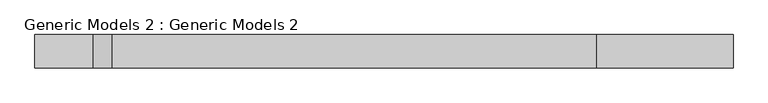
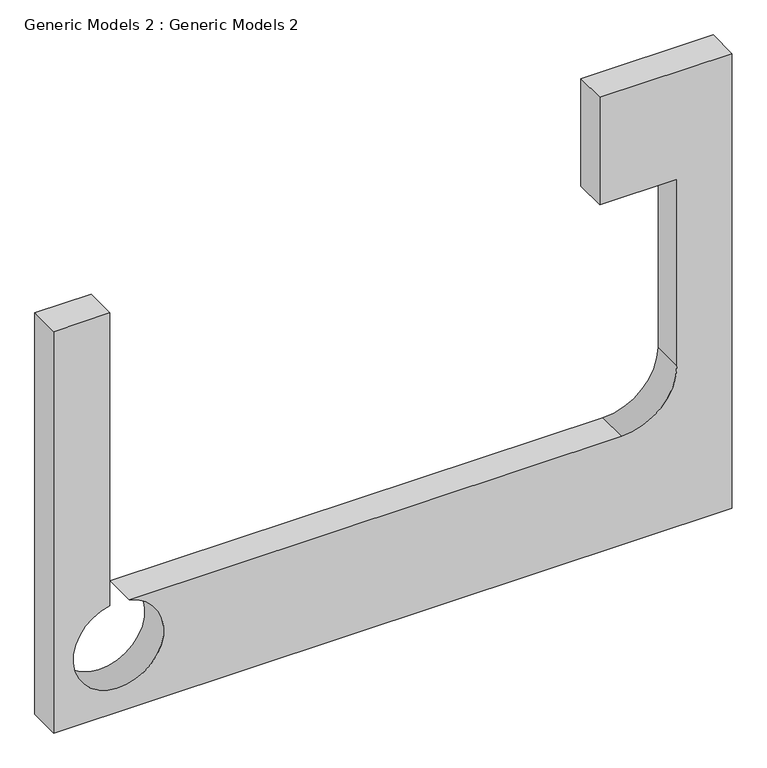
"""IFC4 building model written with IfcOpenShell, lengths in millimetres: proxy geometry, Generic Models 2 : Generic Models 2."""

from ifc_helpers import new_model, si_unit, point, frame, frame_2d, origin, place, context, project, spatial, polyline, circle_curve, trimmed, segment, composite_curve, outline, extrude, source, transform, mapped, element, save


def generic_models_2_generic_models_2_d1d1e900(model_context):
    return source(origin(), model_context, "Body", "SweptSolid", [
        extrude(outline(composite_curve([segment(polyline([(3590.0722399, -13997.6335986), (8094.058524, -13997.6335986), (8094.058524, -15237.8356484), (7030.1491239, -15237.8356484), (7030.1491239, -14513.9356484), (5181.0005, -14513.9356484)]), True, "CONTINUOUS"), segment(trimmed(circle_curve(frame_2d((5181.0005, -15030.2376981)), 516.3020498), [point((5181.0005, -14513.9356484))], [point((4664.6984502, -15030.2376981))], True, "CARTESIAN"), True, "CONTINUOUS"), segment(polyline([(4664.6984502, -15030.2376981), (4664.6984502, -19650.0519369)]), True, "CONTINUOUS"), segment(trimmed(circle_curve(frame_2d((4250.8135385, -19749.3127095)), 425.6212178), [point((4664.6984502, -19650.0519369))], [point((4668.8984575, -19829.0524212))], True, "CARTESIAN"), True, "CONTINUOUS"), segment(polyline([(4668.8984575, -19829.0524212), (7566.4335715, -19829.0524212), (7566.4335715, -20355.9358231), (3590.0722399, -20355.9358231), (3590.0722399, -13997.6335986)]), True, "CONTINUOUS")], self_intersect=False)), frame((0.0, -4597.9088252, 0.0), z_axis=(0.0, 1.0, 0.0), x_axis=(0.0, 0.0, 1.0)), (0.0, 0.0, 1.0), 304.8),
    ])


if __name__ == "__main__":
    model = new_model("IFC4")
    model_context = context("Model", 3, world=origin())
    ifc_project = project(units=[si_unit("LENGTHUNIT", "METRE", prefix="MILLI")], contexts=[model_context])
    site = spatial("IfcSite", under=ifc_project)
    building = spatial("IfcBuilding", under=site)
    placement = place(None, origin())
    generic_models_2_generic_models_2_shape = generic_models_2_generic_models_2_d1d1e900(model_context)
    element("IfcBuildingElementProxy", 1, Name="Generic Models 2 : Generic Models 2", ObjectType="Generic Models 2 : Generic Models 2", at=placement, inside=building, context=model_context, shape_type="MappedRepresentation", body=[
        mapped(generic_models_2_generic_models_2_shape, transform((0.0, 0.0, 0.0), x_axis=(1.0, 0.0, 0.0), y_axis=(0.0, 1.0, 0.0), z_axis=(0.0, 0.0, 1.0))),
    ])
    save(model, "model.ifc")
